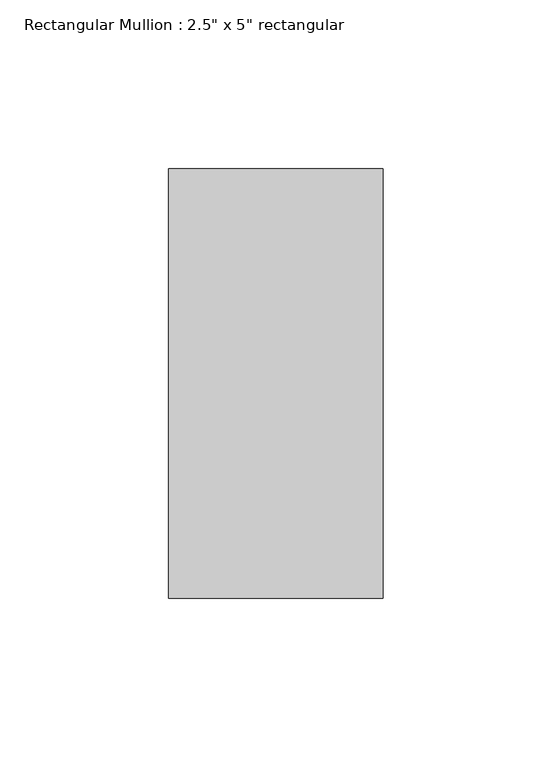
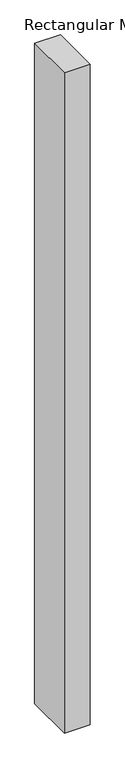
"""IFC4 building model written with IfcOpenShell, lengths in millimetres: member geometry."""

from ifc_helpers import new_model, si_unit, frame, origin, place, context, project, spatial, polyline, outline, extrude, source, transform, mapped, element, save


def member_5ecc8567(model_context):
    return source(origin(), model_context, "Body", "SweptSolid", [
        extrude(outline(polyline([(31.75, 63.5), (31.75, -63.5), (-31.75, -63.5), (-31.75, 63.5), (31.75, 63.5)])), frame((0.0, 0.0, -1728.1374524), z_axis=(0.0, 0.0, 1.0), x_axis=(1.0, 0.0, 0.0)), (0.0, 0.0, 1.0), 1728.1374524),
    ])


if __name__ == "__main__":
    model = new_model("IFC4")
    model_context = context("Model", 3, world=origin())
    ifc_project = project(units=[si_unit("LENGTHUNIT", "METRE", prefix="MILLI")], contexts=[model_context])
    site = spatial("IfcSite", under=ifc_project)
    building = spatial("IfcBuilding", under=site)
    placement = place(None, origin())
    member_shape = member_5ecc8567(model_context)
    element("IfcMember", 1, ObjectType="Rectangular Mullion : 2.5\" x 5\" rectangular", at=placement, inside=building, context=model_context, shape_type="MappedRepresentation", body=[
        mapped(member_shape, transform((0.0, 0.0, 0.0), x_axis=(1.0, 0.0, 0.0), y_axis=(0.0, 1.0, 0.0), z_axis=(0.0, 0.0, 1.0))),
    ])
    save(model, "model.ifc")

# Revit data of these elements
# Type "Rectangular Mullion : 2.5\" x 5\" rectangular"
#   built-in parameter 1007304 = 0.416667 (stored number, unit not read)
#   built-in parameter 1007301 = 0.104167 (stored number, unit not read)
#   built-in parameter 1007300 = 0.104167 (stored number, unit not read)
# Element 1 (IfcMember, "Rectangular Mullion : 2.5\" x 5\" rectangular")
#   Materials on its faces: "Aluminum"
# Materials
#   "Aluminum": class "Metal", colour RGB 247 247 247, transparency 0, Description = "Aluminum 6061", Cost = 0
